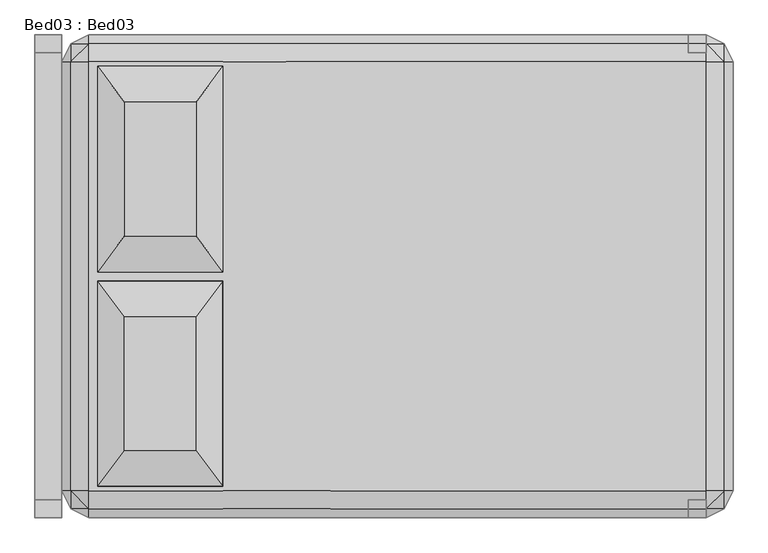
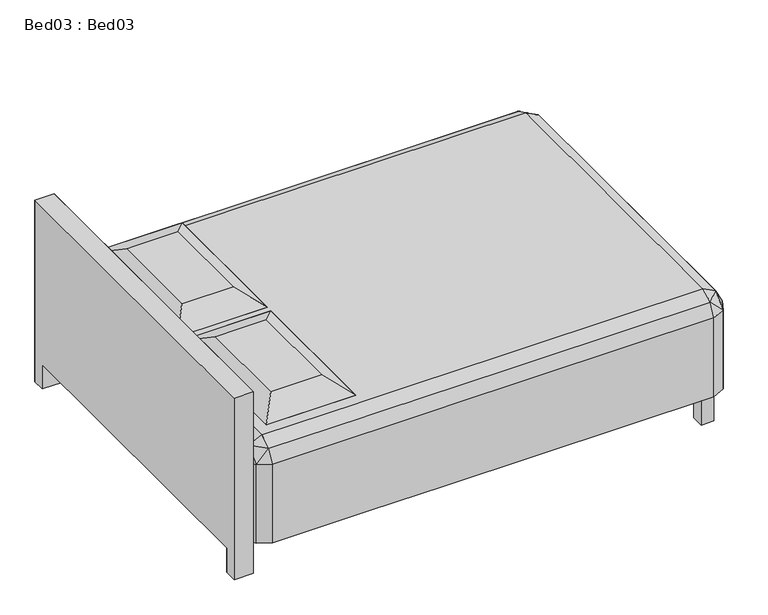
"""IFC4 building model written with IfcOpenShell, lengths in millimetres: furniture geometry, Bed03 : Bed03."""

from ifc_helpers import new_model, si_unit, origin, place, context, project, spatial, triangles, source, transform, mapped, element, save


def bed03_bed03_f6309305(model_context):
    return source(origin(), model_context, "Body", "Tessellation", [
        triangles([(253.9999939, 596.9000121, 507.9999879), (253.9999939, 165.1000061, 508.0000606), (177.7999939, 88.9000151, 533.4000363), (177.7999939, 673.0999758, 533.4), (457.2, 596.9000121, 507.9999879), (533.4, 673.0999758, 533.4), (533.4, 88.9000151, 533.4000363), (457.2, 165.1000061, 508.0000606), (457.2, 571.5, 584.1999879), (253.9999939, 571.5, 584.1999879), (457.2, 190.5000182, 584.2000606), (253.9999939, 190.5000182, 584.2000606), (533.4, 1295.4, 507.9999516), (152.4, 1295.4, 507.9999516), (533.4, 76.2000091, 508.0000606), (152.4, 76.2000091, 508.0000606), (533.4, 25.4000121, 482.6000484), (152.4, 25.4000121, 482.6000484), (533.4, 7.8e-06, 431.8000606), (152.4, 7.8e-06, 431.8000606), (533.4, -2.11e-05, 101.6000575), (152.4, -2.11e-05, 101.6000575), (533.4, 1346.1999516, 482.5999394), (152.4, 1346.1999516, 482.5999394), (533.4, 1371.6, 431.7999516), (152.4, 1371.6, 431.7999516), (533.4, 1371.6, 101.5999394), (152.4, 1371.6, 101.5999394), (711.1999758, 1371.6, 101.5999394), (711.1999758, 1371.6, 431.7999516), (711.1999758, 1346.1999516, 482.5999394), (711.1999758, 1295.4, 507.9999516), (838.2, 25.4000121, 482.6000484), (838.2, 7.8e-06, 431.8000606), (838.2, -2.11e-05, 101.6000575), (838.2, 76.2000091, 508.0000606), (1905.0, 1346.1999516, 482.5999394), (1905.0, 1295.4, 507.9999516), (1930.4000484, 1320.8000484, 482.5999394), (1905.0, 1371.6, 431.7999516), (1955.7999516, 1346.1999516, 431.7999516), (1905.0, 1371.6, 101.5999394), (1955.7999516, 1346.1999516, 101.5999394), (1955.7999516, 1295.4, 482.5999394), (1981.2, 1295.4, 431.7999516), (1981.2, 1295.4, 101.5999485), (1955.7999516, 76.2000091, 482.6000484), (1905.0, 76.2000091, 508.0000606), (1930.4000484, 50.8000106, 482.6000484), (1981.2, 76.2000091, 431.8000606), (1955.7999516, 25.4000098, 431.8000606), (1981.2, 76.1999818, 101.6000484), (1955.7999516, 25.399978, 101.6001575), (1905.0, 25.4000121, 482.6000484), (1905.0, 7.8e-06, 431.8000606), (1905.0, -2.11e-05, 101.6000575), (101.600003, 1295.4, 482.5999394), (126.999997, 1320.8000484, 482.5999394), (76.2, 1295.4, 431.7999516), (101.600003, 1346.1999516, 431.7999516), (76.2, 1295.4, 101.5999485), (101.600003, 1346.1999516, 101.5999394), (126.999997, 50.8000106, 482.6000484), (101.600003, 25.4000098, 431.8000606), (101.600003, 25.399978, 101.6001575), (101.600003, 76.2000091, 482.6000484), (76.2, 76.2000091, 431.8000606), (76.2, 76.1999818, 101.6000484), (253.9999939, 800.1, 584.1999879), (253.9999939, 1181.1, 584.1999516), (177.7999939, 698.5000242, 533.4), (177.7999939, 1282.7000484, 533.3999637), (457.2, 800.1, 584.1999879), (457.2, 1181.1, 584.1999516), (533.4, 1282.7000484, 533.3999637), (533.4, 698.5000242, 533.4), (457.2, 1206.4999758, 507.9999516), (253.9999939, 1206.4999758, 507.9999516), (457.2, 774.7000242, 507.9999879), (253.9999939, 774.7000242, 507.9999879)], [[1, 2, 3], [3, 4, 1], [5, 6, 7], [7, 8, 5], [7, 3, 8], [2, 8, 3], [4, 6, 5], [5, 1, 4], [6, 4, 9], [10, 9, 4], [3, 7, 11], [11, 12, 3], [6, 9, 7], [11, 7, 9], [12, 11, 10], [9, 10, 11], [12, 10, 3], [4, 3, 10], [13, 14, 15], [16, 15, 14], [15, 16, 17], [18, 17, 16], [19, 20, 21], [22, 21, 20], [17, 18, 19], [20, 19, 18], [23, 24, 13], [14, 13, 24], [25, 26, 23], [24, 23, 26], [27, 28, 25], [26, 25, 28], [29, 27, 30], [25, 30, 27], [30, 25, 31], [23, 31, 25], [31, 23, 32], [13, 32, 23], [33, 17, 34], [19, 34, 17], [34, 19, 35], [21, 35, 19], [36, 15, 33], [17, 33, 15], [32, 13, 36], [15, 36, 13], [37, 38, 39], [40, 41, 42], [43, 42, 41], [40, 37, 41], [41, 37, 39], [44, 45, 41], [44, 41, 39], [41, 45, 46], [46, 43, 41], [38, 44, 39], [47, 48, 49], [50, 51, 52], [53, 52, 51], [50, 47, 51], [51, 47, 49], [54, 55, 51], [54, 51, 49], [51, 55, 56], [56, 53, 51], [48, 54, 49], [57, 14, 58], [59, 60, 61], [62, 61, 60], [59, 57, 60], [60, 57, 58], [24, 26, 60], [24, 60, 58], [60, 26, 28], [28, 62, 60], [14, 24, 58], [18, 16, 63], [20, 64, 22], [65, 22, 64], [20, 18, 64], [64, 18, 63], [66, 67, 64], [66, 64, 63], [64, 67, 68], [68, 65, 64], [16, 66, 63], [16, 14, 57], [57, 66, 16], [67, 59, 61], [61, 68, 67], [66, 57, 59], [59, 67, 66], [44, 47, 45], [50, 45, 47], [45, 50, 46], [52, 46, 50], [38, 48, 44], [47, 44, 48], [38, 32, 48], [36, 48, 32], [48, 36, 54], [33, 54, 36], [55, 34, 56], [35, 56, 34], [54, 33, 55], [34, 55, 33], [37, 31, 38], [32, 38, 31], [40, 30, 37], [31, 37, 30], [42, 29, 40], [30, 40, 29], [69, 70, 71], [72, 71, 70], [69, 73, 70], [74, 70, 73], [75, 74, 76], [73, 76, 74], [71, 76, 73], [73, 69, 71], [75, 72, 74], [70, 74, 72], [72, 75, 77], [77, 78, 72], [76, 71, 79], [80, 79, 71], [77, 75, 76], [76, 79, 77], [78, 80, 71], [71, 72, 78]], closed=False),
        triangles([(0.0, 1371.6, 761.9999273), (0.0, 0.0, 762.0000727), (76.2, 1371.6, 761.9999273), (76.2, 0.0, 762.0000727)], [[1, 2, 3], [4, 3, 2]], closed=False),
        triangles([(76.2, 3.33e-05, 762.0000727), (76.2, -2.44e-05, 101.6000575), (76.2, 1371.6, 101.5999394), (76.2, 1371.6, 761.9999273), (1854.2000484, -2.44e-05, 101.6000575), (1854.2000484, -3.33e-05, 6e-05), (1854.2000484, 50.7999743, 101.6001575), (1854.2000484, 50.7999652, 5.55e-05), (1905.0, 50.7999652, 5.55e-05), (1905.0, 50.7999743, 101.6001575), (1905.0, -2.44e-05, 101.6000575), (1905.0, -3.33e-05, 6e-05), (76.2, 50.7999652, 5.55e-05), (76.2, 50.7999743, 101.6001575), (76.2, -3.33e-05, 6e-05), (0.0, -2.44e-05, 101.6000575), (0.0, -3.33e-05, 6e-05), (0.0, 50.7999743, 101.6001575), (0.0, 50.7999652, 5.55e-05), (0.0, 1320.8000484, 101.6000121), (0.0, 1320.8000484, -5.55e-05), (0.0, 1371.6, 101.5999394), (0.0, 1371.6, -6e-05), (76.2, 1371.6, -6e-05), (76.2, 1320.8000484, 101.6000121), (76.2, 1320.8000484, -5.55e-05), (1905.0, 1371.6, -6e-05), (1905.0, 1371.6, 101.5999394), (1905.0, 1320.8000484, 101.6000121), (1905.0, 1320.8000484, -5.55e-05), (1854.2000484, 1320.8000484, 101.6000121), (1854.2000484, 1320.8000484, -5.55e-05), (1854.2000484, 1371.6, 101.5999394), (1854.2000484, 1371.6, -6e-05), (0.0, 3.33e-05, 762.0000727), (0.0, 1371.6, 761.9999273)], [[1, 2, 3], [3, 4, 1], [5, 6, 7], [8, 7, 6], [9, 10, 11], [11, 12, 9], [13, 14, 2], [2, 15, 13], [16, 17, 18], [19, 18, 17], [20, 21, 22], [23, 22, 21], [24, 3, 25], [25, 26, 24], [27, 28, 29], [29, 30, 27], [31, 32, 33], [34, 33, 32], [35, 16, 36], [22, 36, 16]], closed=False),
        triangles([(76.2, 3.33e-05, 762.0000727), (76.2, -2.44e-05, 101.6000575), (0.0, -2.44e-05, 101.6000575), (76.2, 1371.6, 761.9999273), (76.2, 1371.6, 101.5999394), (0.0, 1371.6, 761.9999273), (0.0, 1371.6, 101.5999394), (0.0, -3.33e-05, 6e-05), (76.2, -3.33e-05, 6e-05), (76.2, 50.7999743, 101.6001575), (76.2, 50.7999652, 5.55e-05), (0.0, 50.7999743, 101.6001575), (0.0, 50.7999652, 5.55e-05), (76.2, 1371.6, -6e-05), (0.0, 1371.6, -6e-05), (0.0, 1320.8000484, -5.55e-05), (0.0, 1320.8000484, 101.6000121), (76.2, 1320.8000484, 101.6000121), (76.2, 1320.8000484, -5.55e-05), (1854.2000484, -3.33e-05, 6e-05), (1854.2000484, -2.44e-05, 101.6000575), (1905.0, -2.44e-05, 101.6000575), (1905.0, -3.33e-05, 6e-05), (1905.0, 50.7999743, 101.6001575), (1905.0, 50.7999652, 5.55e-05), (1854.2000484, 50.7999743, 101.6001575), (1854.2000484, 50.7999652, 5.55e-05), (1854.2000484, 1320.8000484, -5.55e-05), (1854.2000484, 1320.8000484, 101.6000121), (1905.0, 1320.8000484, 101.6000121), (1905.0, 1320.8000484, -5.55e-05), (1905.0, 1371.6, 101.5999394), (1905.0, 1371.6, -6e-05), (1854.2000484, 1371.6, 101.5999394), (1854.2000484, 1371.6, -6e-05), (0.0, 3.33e-05, 762.0000727)], [[1, 2, 3], [4, 5, 6], [7, 6, 5], [8, 3, 2], [2, 9, 8], [10, 11, 12], [13, 12, 11], [5, 14, 7], [15, 7, 14], [16, 17, 18], [18, 19, 16], [20, 21, 22], [22, 23, 20], [24, 25, 26], [27, 26, 25], [28, 29, 30], [30, 31, 28], [32, 33, 34], [35, 34, 33], [3, 36, 1]], closed=False),
    ])


if __name__ == "__main__":
    model = new_model("IFC4")
    model_context = context("Model", 3, world=origin())
    ifc_project = project(units=[si_unit("LENGTHUNIT", "METRE", prefix="MILLI")], contexts=[model_context])
    site = spatial("IfcSite", under=ifc_project)
    building = spatial("IfcBuilding", under=site)
    placement = place(None, origin())
    bed03_bed03_shape = bed03_bed03_f6309305(model_context)
    element("IfcFurniture", 1, ObjectType="Bed03 : Bed03", at=placement, inside=building, context=model_context, shape_type="MappedRepresentation", body=[
        mapped(bed03_bed03_shape, transform((0.0, 0.0, 0.0), x_axis=(1.0, 0.0, 0.0), y_axis=(0.0, 1.0, 0.0), z_axis=(0.0, 0.0, 1.0))),
    ])
    save(model, "model.ifc")

# Revit data of these elements
# Type "Bed03 : Bed03"
#   Default Elevation = 0
